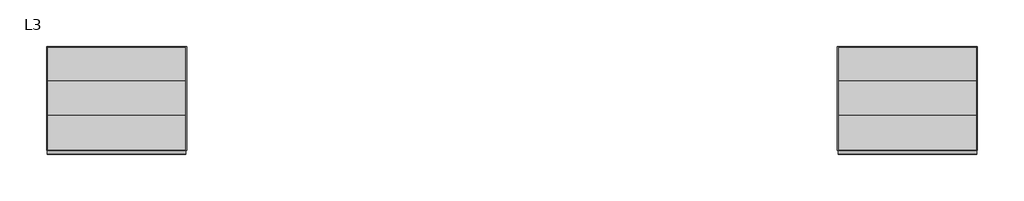
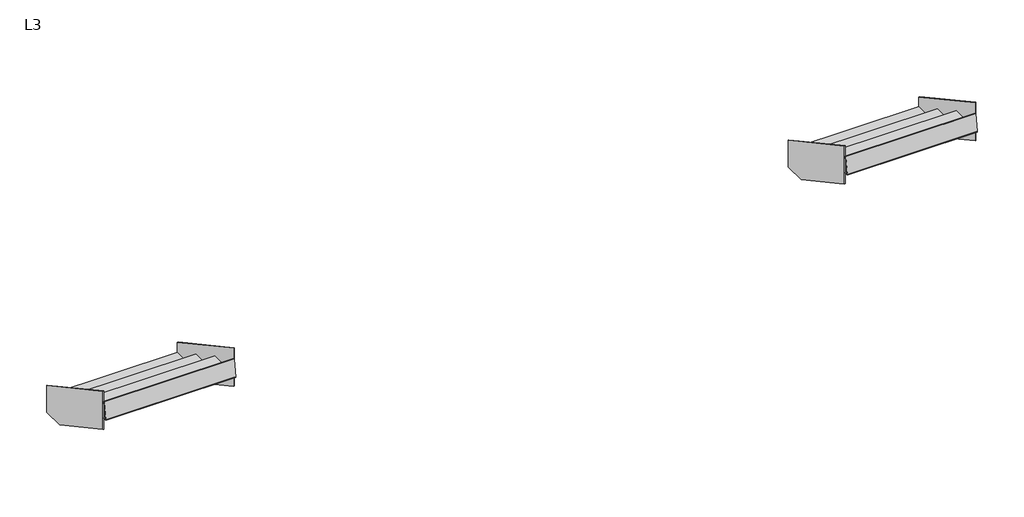
# One storey: 4 members, 2 stair flights.
"""IFC4 building model written with IfcOpenShell, lengths in millimetres."""

from ifc_helpers import new_model, si_unit, frame, origin, place, context, project, spatial, polyline, outline, extrude, transform, mapped, element, save
from components import stair_flight_a16d44b4, stair_flight_307daca0

model = new_model("IFC4")

# Units and contexts
model_context = context("Model", 3, world=origin())
ifc_project = project(units=[si_unit("LENGTHUNIT", "METRE", prefix="MILLI")], contexts=[model_context])

# Site, building, storey
site = spatial("IfcSite", under=ifc_project)
building = spatial("IfcBuilding", under=site)
storey = spatial("IfcBuildingStorey", under=building, Name="L3", Elevation=0.0)

# Members
placement = place(None, origin())
element("IfcMember", 1, ObjectType="Stringer - 1/4\" Plate", at=placement, inside=storey, context=model_context, shape_type="SweptSolid", body=[
    extrude(outline(polyline([(6287.0278379, 241.8661658), (6287.0278379, 0.0), (6093.9269663, 0.0), (5448.8278379, 351.8722519), (5448.8278379, 699.0661658), (6287.0278379, 241.8661658)])), frame((-791.4879185, 0.0, 0.0), z_axis=(1.0, 0.0, 0.0), x_axis=(0.0, 1.0, 0.0)), (0.0, 0.0, 1.0), 6.35),
])
element("IfcMember", 2, ObjectType="Stringer - 1/4\" Plate", at=placement, inside=storey, context=model_context, shape_type="SweptSolid", body=[
    extrude(outline(polyline([(6287.0278379, 241.8661658), (6287.0278379, 0.0), (6093.9269663, 0.0), (5448.8278379, 351.8722519), (5448.8278379, 699.0661658), (6287.0278379, 241.8661658)])), frame((-1915.4379185, 0.0, 0.0), z_axis=(1.0, 0.0, 0.0), x_axis=(0.0, 1.0, 0.0)), (0.0, 0.0, 1.0), 6.35),
])
element("IfcMember", 3, ObjectType="Stringer - 1/4\" Plate", at=placement, inside=storey, context=model_context, shape_type="SweptSolid", body=[
    extrude(outline(polyline([(6287.0278379, 241.8661658), (6287.0278379, 0.0), (6093.9269663, 0.0), (5448.8278379, 351.8722519), (5448.8278379, 699.0661658), (6287.0278379, 241.8661658)])), frame((5583.9120815, 0.0, 0.0), z_axis=(1.0, 0.0, 0.0), x_axis=(0.0, 1.0, 0.0)), (0.0, 0.0, 1.0), 6.35),
])
element("IfcMember", 4, ObjectType="Stringer - 1/4\" Plate", at=placement, inside=storey, context=model_context, shape_type="SweptSolid", body=[
    extrude(outline(polyline([(6287.0278379, 241.8661658), (6287.0278379, 0.0), (6093.9269663, 0.0), (5448.8278379, 351.8722519), (5448.8278379, 699.0661658), (6287.0278379, 241.8661658)])), frame((4459.9620815, 0.0, 0.0), z_axis=(1.0, 0.0, 0.0), x_axis=(0.0, 1.0, 0.0)), (0.0, 0.0, 1.0), 6.35),
])

# Stair flights
stair_flight_shape = stair_flight_a16d44b4(model_context)
element("IfcStairFlight", 5, ObjectType="1/4\" Tread 1\" Nosing 1/4\" Riser", at=placement, inside=storey, context=model_context, shape_type="MappedRepresentation", body=[
    mapped(stair_flight_shape, transform((0.0, 0.0, 0.0), x_axis=(1.0, 0.0, 0.0), y_axis=(0.0, 1.0, 0.0), z_axis=(0.0, 0.0, 1.0))),
])
stair_flight_2_shape = stair_flight_307daca0(model_context)
element("IfcStairFlight", 6, ObjectType="1/4\" Tread 1\" Nosing 1/4\" Riser", at=placement, inside=storey, context=model_context, shape_type="MappedRepresentation", body=[
    mapped(stair_flight_2_shape, transform((0.0, 0.0, 0.0), x_axis=(1.0, 0.0, 0.0), y_axis=(0.0, 1.0, 0.0), z_axis=(0.0, 0.0, 1.0))),
])

save(model, "model.ifc")

# Revit data of these elements
# Elements 1, 2, 3, 4 (IfcMember, "Stringer - 1/4\" Plate")
#   Phase Created = New Construction
#   Materials on its faces: "Steel, Paint Finish, Dark Gray"
# Elements 5, 6 (IfcStairFlight, "1/4\" Tread 1\" Nosing 1/4\" Riser")
#   Phase Created = New Construction
#   Materials on its faces: "Steel, Paint Finish, Dark Gray"
# Materials
#   "Steel, Paint Finish, Dark Gray": class "Metal", colour RGB 89 89 89, transparency 0, Description = "Steel, paint finish, dark gray, glossy", Cost = 0
